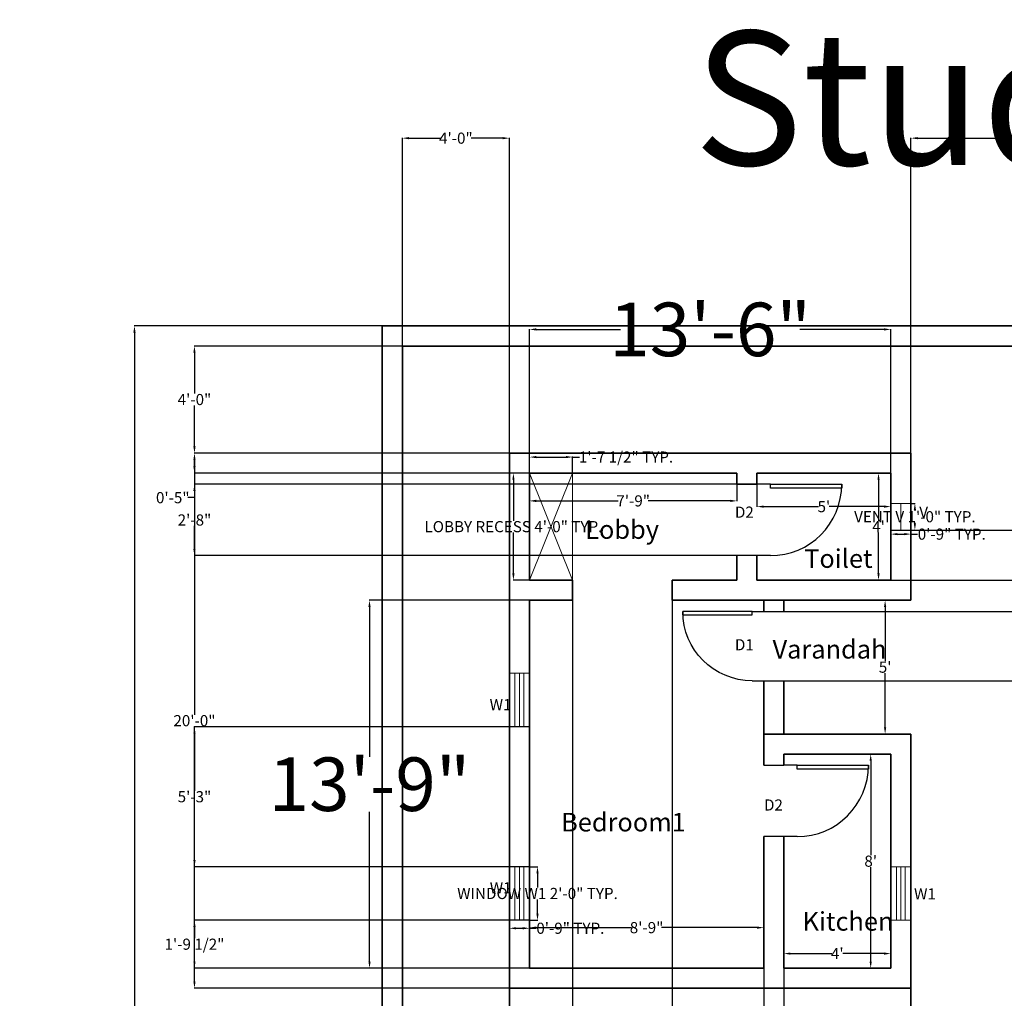
# Model space of a CAD drawing. Units: inches. Extents: x -205 to 674, y 63 to 1798.
# Tile 3 of 4: x -205 to 236, y 1359 to 1798. Entities that reach past the tile are written whole.
import ezdxf

# ---------------------------------------------------------------- set-up
doc = ezdxf.new("R2010")
doc.units = ezdxf.units.IN
doc.header["$MEASUREMENT"] = 0
doc.layers.get('0').update_dxf_attribs({"color": 70})
for name, color, linetype, lineweight in [('A-ANNO-DIMS', 240, 'Continuous', 18), ('A-ANNO-TEXT', 240, 'Continuous', 18), ('A-AREA-IDEN', 240, 'Continuous', 18), ('A-WALL', 70, 'Continuous', 35), ('A-WALL-SITE', 70, 'Continuous', 35), ('door1', 20, 'Continuous', 25), ('door2', 160, 'Continuous', 25), ('lobby', 241, 'Continuous', 18), ('ventilator1', 210, 'Continuous', 18), ('window1', 50, 'Continuous', 18)]:
    doc.layers.add(name, color=color, linetype=linetype, lineweight=lineweight)
doc.styles.get("Standard").update_dxf_attribs({"font": 'arial.ttf'})
doc.dimstyles.get("Standard").update_dxf_attribs({"dimtxt": 5, "dimasz": 3, "dimexe": 0.18, "dimexo": 0.0625, "dimgap": 0.09, "dimtad": 0, "dimtih": 1, "dimtoh": 1, "dimdec": 0, "dimzin": 0, "dimdsep": 46, "dimlunit": 3, "dimtxsty": 'Standard', "dimcen": 0.09, "dimadec": 0, "dimazin": 0, "dimtfac": 1, "dimtdec": 0, "dimtofl": 0, "dimtmove": 0, "dimatfit": 3, "dimfxl": 1, "dimtolj": 1, "dimtzin": 0, "dimarcsym": 0})

# ---------------------------------------------------------------- blocks, each defined once
blk = doc.blocks.new('*D1')
at = {"layer": 'A-ANNO-DIMS', "color": 0, "lineweight": -2, "transparency": 16777216}
for p, q in [((23.48, 1537.3), (-48.36, 1537.3)), ((-48.18, 1534.3), (-48.18, 1467.15)), ((-48.18, 1375.3), (-48.18, 1442.45)), ((23.48, 1372.3), (-48.36, 1372.3))]:
    blk.add_line(p, q, dxfattribs=at)
at = {"layer": 'A-ANNO-DIMS', "color": 0, "transparency": 16777216}
for points in [[(-48.68, 1534.3), (-47.68, 1534.3), (-48.18, 1537.3)], [(-48.68, 1375.3), (-47.68, 1375.3), (-48.18, 1372.3)]]:
    blk.add_solid(points, dxfattribs=at)
at = {"layer": 'Defpoints', "color": 0, "transparency": 16777216}
for p in [(23.54, 1537.3), (-48.18, 1372.3), (23.54, 1372.3)]:
    blk.add_point(p, dxfattribs=at)
at = {"layer": 'A-ANNO-DIMS', "color": 0, "transparency": 16777216, "insert": (-48.18, 1454.8), "char_height": 5, "attachment_point": 5}
blk.add_mtext('\\A1;{\\H4.8x;13\'-9"}', dxfattribs=at)
blk = doc.blocks.new('*D2')
at = {"layer": 'A-ANNO-DIMS', "color": 0, "lineweight": -2, "transparency": 16777216}
for p, q in [((23.54, 1594.36), (23.54, 1658.92)), ((26.54, 1658.74), (64.36, 1658.74)), ((182.54, 1658.74), (144.73, 1658.74)), ((185.54, 1594.36), (185.54, 1658.92))]:
    blk.add_line(p, q, dxfattribs=at)
at = {"layer": 'A-ANNO-DIMS', "color": 0, "transparency": 16777216}
for points in [[(26.54, 1659.24), (26.54, 1658.24), (23.54, 1658.74)], [(182.54, 1659.24), (182.54, 1658.24), (185.54, 1658.74)]]:
    blk.add_solid(points, dxfattribs=at)
at = {"layer": 'Defpoints', "color": 0, "transparency": 16777216}
for p in [(185.54, 1658.74), (23.54, 1594.3), (185.54, 1594.3)]:
    blk.add_point(p, dxfattribs=at)
at = {"layer": 'A-ANNO-DIMS', "color": 0, "transparency": 16777216, "insert": (104.54, 1658.74), "char_height": 5, "attachment_point": 5}
blk.add_mtext('\\A1;{\\H4.8x;13\'-6"}', dxfattribs=at)
blk = doc.blocks.new('*U4')
for p, q in [((0, 0), (0, -6)), ((36, 0), (36, -6))]:
    blk.add_line(p, q)
blk.add_lwpolyline([(0, 0), (0, 36), (1.75, 36), (1.75, 0)], close=True)
blk.add_arc((0, 0), 36, 0, 90)
blk = doc.blocks.new('*U5')
for p, q in [((0, 0), (0, -6)), ((32, 0), (32, -6))]:
    blk.add_line(p, q)
blk.add_lwpolyline([(0, 0), (0, 32), (1.75, 32), (1.75, 0)], close=True)
blk.add_arc((0, 0), 32, 0, 90)
blk = doc.blocks.new('*D18')
at = {"layer": 'A-ANNO-DIMS', "color": 0, "lineweight": -2, "transparency": 16777216}
for p, q in [((-42.52, 1660.3), (-153.74, 1660.3)), ((-153.56, 1657.3), (-153.56, 919.64)), ((-153.56, 157.3), (-153.56, 894.96)), ((-42.52, 154.3), (-153.74, 154.3))]:
    blk.add_line(p, q, dxfattribs=at)
at = {"layer": 'A-ANNO-DIMS', "color": 0, "transparency": 16777216}
for points in [[(-154.06, 1657.3), (-153.06, 1657.3), (-153.56, 1660.3)], [(-154.06, 157.3), (-153.06, 157.3), (-153.56, 154.3)]]:
    blk.add_solid(points, dxfattribs=at)
at = {"layer": 'Defpoints', "color": 0, "transparency": 16777216}
for p in [(-42.46, 1660.3), (-153.56, 154.3), (-42.46, 154.3)]:
    blk.add_point(p, dxfattribs=at)
at = {"layer": 'A-ANNO-DIMS', "color": 0, "transparency": 16777216, "insert": (-153.56, 907.3), "char_height": 5, "attachment_point": 5}
blk.add_mtext('\\A1;{\\H4.8x;125\'-6"}', dxfattribs=at)
blk = doc.blocks.new('*D20')
at = {"layer": 'A-ANNO-DIMS', "color": 0, "lineweight": -2, "transparency": 16777216}
for p, q in [((23.54, 1372.36), (23.54, 1390.67)), ((128.54, 1372.36), (128.54, 1390.67)), ((26.54, 1390.49), (69.3, 1390.49)), ((125.54, 1390.49), (82.78, 1390.49))]:
    blk.add_line(p, q, dxfattribs=at)
at = {"layer": 'A-ANNO-DIMS', "color": 0, "transparency": 16777216}
for points in [[(26.54, 1390.99), (26.54, 1389.99), (23.54, 1390.49)], [(125.54, 1390.99), (125.54, 1389.99), (128.54, 1390.49)]]:
    blk.add_solid(points, dxfattribs=at)
at = {"layer": 'Defpoints', "color": 0, "transparency": 16777216}
for p in [(128.54, 1390.49), (23.54, 1372.3), (128.54, 1372.3)]:
    blk.add_point(p, dxfattribs=at)
at = {"layer": 'A-ANNO-DIMS', "color": 0, "transparency": 16777216, "insert": (76.04, 1390.49), "char_height": 5, "attachment_point": 5}
blk.add_mtext('\\A1;8\'-9"', dxfattribs=at)
blk = doc.blocks.new('*D21')
at = {"layer": 'A-ANNO-DIMS', "color": 0, "lineweight": -2, "transparency": 16777216}
for p, q in [((137.54, 1372.36), (137.54, 1379.04)), ((140.54, 1378.86), (159.05, 1378.86)), ((182.54, 1378.86), (164.03, 1378.86)), ((185.54, 1372.36), (185.54, 1379.04))]:
    blk.add_line(p, q, dxfattribs=at)
at = {"layer": 'A-ANNO-DIMS', "color": 0, "transparency": 16777216}
for points in [[(140.54, 1379.36), (140.54, 1378.36), (137.54, 1378.86)], [(182.54, 1379.36), (182.54, 1378.36), (185.54, 1378.86)]]:
    blk.add_solid(points, dxfattribs=at)
at = {"layer": 'Defpoints', "color": 0, "transparency": 16777216}
for p in [(185.54, 1378.86), (137.54, 1372.3), (185.54, 1372.3)]:
    blk.add_point(p, dxfattribs=at)
at = {"layer": 'A-ANNO-DIMS', "color": 0, "transparency": 16777216, "insert": (161.54, 1378.86), "char_height": 5, "attachment_point": 5}
blk.add_mtext("\\A1;4'", dxfattribs=at)
blk = doc.blocks.new('*D22')
at = {"layer": 'A-ANNO-DIMS', "color": 0, "lineweight": -2, "transparency": 16777216}
for p, q in [((185.48, 1468.3), (176.35, 1468.3)), ((176.53, 1465.3), (176.53, 1422.94)), ((176.53, 1375.3), (176.53, 1417.66)), ((185.48, 1372.3), (176.35, 1372.3))]:
    blk.add_line(p, q, dxfattribs=at)
at = {"layer": 'A-ANNO-DIMS', "color": 0, "transparency": 16777216}
for points in [[(176.03, 1465.3), (177.03, 1465.3), (176.53, 1468.3)], [(176.03, 1375.3), (177.03, 1375.3), (176.53, 1372.3)]]:
    blk.add_solid(points, dxfattribs=at)
at = {"layer": 'Defpoints', "color": 0, "transparency": 16777216}
for p in [(185.54, 1468.3), (176.53, 1372.3), (185.54, 1372.3)]:
    blk.add_point(p, dxfattribs=at)
at = {"layer": 'A-ANNO-DIMS', "color": 0, "transparency": 16777216, "insert": (176.53, 1420.3), "char_height": 5, "attachment_point": 5}
blk.add_mtext("\\A1;8'", dxfattribs=at)
blk = doc.blocks.new('*D23')
at = {"layer": 'A-ANNO-DIMS', "color": 0, "lineweight": -2, "transparency": 16777216}
for p, q in [((185.48, 1594.3), (179.86, 1594.3)), ((180.04, 1591.3), (180.04, 1572.89)), ((180.04, 1549.3), (180.04, 1567.71)), ((185.48, 1546.3), (179.86, 1546.3))]:
    blk.add_line(p, q, dxfattribs=at)
at = {"layer": 'A-ANNO-DIMS', "color": 0, "transparency": 16777216}
for points in [[(179.54, 1591.3), (180.54, 1591.3), (180.04, 1594.3)], [(179.54, 1549.3), (180.54, 1549.3), (180.04, 1546.3)]]:
    blk.add_solid(points, dxfattribs=at)
at = {"layer": 'Defpoints', "color": 0, "transparency": 16777216}
for p in [(185.54, 1594.3), (180.04, 1546.3), (185.54, 1546.3)]:
    blk.add_point(p, dxfattribs=at)
at = {"layer": 'A-ANNO-DIMS', "color": 0, "transparency": 16777216, "insert": (180.04, 1570.3), "char_height": 5, "attachment_point": 5}
blk.add_mtext("\\A1;4'", dxfattribs=at)
blk = doc.blocks.new('*D24')
at = {"layer": 'A-ANNO-DIMS', "color": 0, "lineweight": -2, "transparency": 16777216}
for p, q in [((125.54, 1594.24), (125.54, 1579.11)), ((185.54, 1594.24), (185.54, 1579.11)), ((128.54, 1579.29), (153.15, 1579.29)), ((182.54, 1579.29), (157.93, 1579.29))]:
    blk.add_line(p, q, dxfattribs=at)
at = {"layer": 'A-ANNO-DIMS', "color": 0, "transparency": 16777216}
for points in [[(128.54, 1579.79), (128.54, 1578.79), (125.54, 1579.29)], [(182.54, 1579.79), (182.54, 1578.79), (185.54, 1579.29)]]:
    blk.add_solid(points, dxfattribs=at)
at = {"layer": 'Defpoints', "color": 0, "transparency": 16777216}
for p in [(125.54, 1594.3), (185.54, 1594.3), (125.54, 1579.29)]:
    blk.add_point(p, dxfattribs=at)
at = {"layer": 'A-ANNO-DIMS', "color": 0, "transparency": 16777216, "insert": (155.54, 1579.29), "char_height": 5, "attachment_point": 5}
blk.add_mtext("\\A1;5'", dxfattribs=at)
blk = doc.blocks.new('*D25')
at = {"layer": 'A-ANNO-DIMS', "color": 0, "lineweight": -2, "transparency": 16777216}
for p, q in [((23.54, 1594.24), (23.54, 1581.67)), ((116.54, 1594.24), (116.54, 1581.67)), ((26.54, 1581.85), (63.33, 1581.85)), ((113.54, 1581.85), (76.76, 1581.85))]:
    blk.add_line(p, q, dxfattribs=at)
at = {"layer": 'A-ANNO-DIMS', "color": 0, "transparency": 16777216}
for points in [[(26.54, 1582.35), (26.54, 1581.35), (23.54, 1581.85)], [(113.54, 1582.35), (113.54, 1581.35), (116.54, 1581.85)]]:
    blk.add_solid(points, dxfattribs=at)
at = {"layer": 'Defpoints', "color": 0, "transparency": 16777216}
for p in [(23.54, 1594.3), (116.54, 1594.3), (23.54, 1581.85)]:
    blk.add_point(p, dxfattribs=at)
at = {"layer": 'A-ANNO-DIMS', "color": 0, "transparency": 16777216, "insert": (70.04, 1581.85), "char_height": 5, "attachment_point": 5}
blk.add_mtext('\\A1;7\'-9"', dxfattribs=at)
blk = doc.blocks.new('*D26')
at = {"layer": 'A-ANNO-DIMS', "color": 0, "lineweight": -2, "transparency": 16777216}
for p, q in [((194.48, 1537.3), (182.81, 1537.3)), ((182.99, 1534.3), (182.99, 1509.93)), ((182.99, 1480.3), (182.99, 1504.67)), ((194.48, 1477.3), (182.81, 1477.3))]:
    blk.add_line(p, q, dxfattribs=at)
at = {"layer": 'A-ANNO-DIMS', "color": 0, "transparency": 16777216}
for points in [[(182.49, 1534.3), (183.49, 1534.3), (182.99, 1537.3)], [(182.49, 1480.3), (183.49, 1480.3), (182.99, 1477.3)]]:
    blk.add_solid(points, dxfattribs=at)
at = {"layer": 'Defpoints', "color": 0, "transparency": 16777216}
for p in [(194.54, 1537.3), (182.99, 1477.3), (194.54, 1477.3)]:
    blk.add_point(p, dxfattribs=at)
at = {"layer": 'A-ANNO-DIMS', "color": 0, "transparency": 16777216, "insert": (182.99, 1507.3), "char_height": 5, "attachment_point": 5}
blk.add_mtext("\\A1;5'", dxfattribs=at)
blk = doc.blocks.new('WIN-W1-24IN')
for p, q in [((2.5, 24), (2.5, 0)), ((4.5, 24), (4.5, 0)), ((6.5, 24), (6.5, 0))]:
    blk.add_line(p, q)
blk.add_lwpolyline([(0, 24), (9, 24), (9, 0), (0, 0)], close=True)
blk = doc.blocks.new('VENT-V-12IN')
blk.add_line((4.5, 12), (4.5, 0))
blk.add_lwpolyline([(9, 0), (0, 0), (0, 12), (9, 12)], close=True)
blk = doc.blocks.new('LOBBY-RECESS')
for p, q in [((0, 48), (19.36, 0)), ((0, 0), (19.36, 48)), ((19.36, 48), (19.36, 0))]:
    blk.add_line(p, q)
blk = doc.blocks.new('*D30')
at = {"layer": 'A-ANNO-DIMS', "color": 0, "lineweight": -2, "transparency": 16777216}
for p, q in [((23.6, 1417.81), (27.32, 1417.81)), ((27.14, 1414.81), (27.14, 1408.49)), ((27.14, 1396.81), (27.14, 1403.13)), ((23.6, 1393.81), (27.32, 1393.81))]:
    blk.add_line(p, q, dxfattribs=at)
at = {"layer": 'A-ANNO-DIMS', "color": 0, "transparency": 16777216}
for points in [[(26.64, 1414.81), (27.64, 1414.81), (27.14, 1417.81)], [(26.64, 1396.81), (27.64, 1396.81), (27.14, 1393.81)]]:
    blk.add_solid(points, dxfattribs=at)
at = {"layer": 'Defpoints', "color": 0, "transparency": 16777216}
for p in [(23.54, 1417.81), (27.14, 1417.81), (23.54, 1393.81)]:
    blk.add_point(p, dxfattribs=at)
at = {"layer": 'A-ANNO-DIMS', "color": 0, "transparency": 16777216, "insert": (27.14, 1405.81), "char_height": 5, "attachment_point": 5}
blk.add_mtext('\\A1;WINDOW W1 2\'-0" TYP.', dxfattribs=at)
blk = doc.blocks.new('*D31')
at = {"layer": 'A-ANNO-DIMS', "color": 0, "lineweight": -2, "transparency": 16777216}
for p, q in [((14.54, 1393.75), (14.54, 1390.03)), ((23.54, 1393.75), (23.54, 1390.03)), ((17.54, 1390.21), (20.54, 1390.21)), ((23.54, 1390.21), (26.54, 1390.21))]:
    blk.add_line(p, q, dxfattribs=at)
at = {"layer": 'A-ANNO-DIMS', "color": 0, "transparency": 16777216}
for points in [[(17.54, 1390.71), (17.54, 1389.71), (14.54, 1390.21)], [(20.54, 1390.71), (20.54, 1389.71), (23.54, 1390.21)]]:
    blk.add_solid(points, dxfattribs=at)
at = {"layer": 'Defpoints', "color": 0, "transparency": 16777216}
for p in [(14.54, 1393.81), (23.54, 1393.81), (23.54, 1390.21)]:
    blk.add_point(p, dxfattribs=at)
at = {"layer": 'A-ANNO-DIMS', "color": 0, "transparency": 16777216, "insert": (41.87, 1390.21), "char_height": 5, "attachment_point": 5}
blk.add_mtext('\\A1;0\'-9" TYP.', dxfattribs=at)
blk = doc.blocks.new('*D32')
at = {"layer": 'A-ANNO-DIMS', "color": 0, "lineweight": -2, "transparency": 16777216}
for p, q in [((194.6, 1580.75), (196.52, 1580.75)), ((196.34, 1577.75), (196.34, 1577.4)), ((196.34, 1571.75), (196.34, 1572.11)), ((194.6, 1568.75), (196.52, 1568.75))]:
    blk.add_line(p, q, dxfattribs=at)
at = {"layer": 'A-ANNO-DIMS', "color": 0, "transparency": 16777216}
for points in [[(195.84, 1577.75), (196.84, 1577.75), (196.34, 1580.75)], [(195.84, 1571.75), (196.84, 1571.75), (196.34, 1568.75)]]:
    blk.add_solid(points, dxfattribs=at)
at = {"layer": 'Defpoints', "color": 0, "transparency": 16777216}
for p in [(194.54, 1580.75), (196.34, 1580.75), (194.54, 1568.75)]:
    blk.add_point(p, dxfattribs=at)
at = {"layer": 'A-ANNO-DIMS', "color": 0, "transparency": 16777216, "insert": (196.34, 1574.75), "char_height": 5, "attachment_point": 5}
blk.add_mtext('\\A1;VENT V 1\'-0" TYP.', dxfattribs=at)
blk = doc.blocks.new('*D33')
at = {"layer": 'A-ANNO-DIMS', "color": 0, "lineweight": -2, "transparency": 16777216}
for p, q in [((185.54, 1568.69), (185.54, 1566.77)), ((194.54, 1568.69), (194.54, 1566.77)), ((188.54, 1566.95), (191.54, 1566.95)), ((194.54, 1566.95), (197.54, 1566.95))]:
    blk.add_line(p, q, dxfattribs=at)
at = {"layer": 'A-ANNO-DIMS', "color": 0, "transparency": 16777216}
for points in [[(188.54, 1567.45), (188.54, 1566.45), (185.54, 1566.95)], [(191.54, 1567.45), (191.54, 1566.45), (194.54, 1566.95)]]:
    blk.add_solid(points, dxfattribs=at)
at = {"layer": 'Defpoints', "color": 0, "transparency": 16777216}
for p in [(185.54, 1568.75), (194.54, 1568.75), (194.54, 1566.95)]:
    blk.add_point(p, dxfattribs=at)
at = {"layer": 'A-ANNO-DIMS', "color": 0, "transparency": 16777216, "insert": (212.87, 1566.95), "char_height": 5, "attachment_point": 5}
blk.add_mtext('\\A1;0\'-9" TYP.', dxfattribs=at)
blk = doc.blocks.new('*D34')
at = {"layer": 'A-ANNO-DIMS', "color": 0, "lineweight": -2, "transparency": 16777216}
for p, q in [((23.48, 1594.3), (16.16, 1594.3)), ((16.34, 1591.3), (16.34, 1572.98)), ((16.34, 1549.3), (16.34, 1567.62)), ((23.48, 1546.3), (16.16, 1546.3))]:
    blk.add_line(p, q, dxfattribs=at)
at = {"layer": 'A-ANNO-DIMS', "color": 0, "transparency": 16777216}
for points in [[(15.84, 1591.3), (16.84, 1591.3), (16.34, 1594.3)], [(15.84, 1549.3), (16.84, 1549.3), (16.34, 1546.3)]]:
    blk.add_solid(points, dxfattribs=at)
at = {"layer": 'Defpoints', "color": 0, "transparency": 16777216}
for p in [(16.34, 1594.3), (23.54, 1594.3), (23.54, 1546.3)]:
    blk.add_point(p, dxfattribs=at)
at = {"layer": 'A-ANNO-DIMS', "color": 0, "transparency": 16777216, "insert": (16.34, 1570.3), "char_height": 5, "attachment_point": 5}
blk.add_mtext('\\A1;LOBBY RECESS 4\'-0" TYP.', dxfattribs=at)
blk = doc.blocks.new('*D35')
at = {"layer": 'A-ANNO-DIMS', "color": 0, "lineweight": -2, "transparency": 16777216}
for p, q in [((23.54, 1594.36), (23.54, 1601.68)), ((26.54, 1601.5), (39.9, 1601.5)), ((42.9, 1594.36), (42.9, 1601.68)), ((42.9, 1601.5), (45.9, 1601.5))]:
    blk.add_line(p, q, dxfattribs=at)
at = {"layer": 'A-ANNO-DIMS', "color": 0, "transparency": 16777216}
for points in [[(26.54, 1602), (26.54, 1601), (23.54, 1601.5)], [(39.9, 1602), (39.9, 1601), (42.9, 1601.5)]]:
    blk.add_solid(points, dxfattribs=at)
at = {"layer": 'Defpoints', "color": 0, "transparency": 16777216}
for p in [(42.9, 1601.5), (23.54, 1594.3), (42.9, 1594.3)]:
    blk.add_point(p, dxfattribs=at)
at = {"layer": 'A-ANNO-DIMS', "color": 0, "transparency": 16777216, "insert": (66.82, 1601.5), "char_height": 5, "attachment_point": 5}
blk.add_mtext('\\A1;1\'-7 1/2" TYP.', dxfattribs=at)
blk = doc.blocks.new('*D36')
at = {"layer": 'A-ANNO-DIMS', "color": 0, "lineweight": -2, "transparency": 16777216}
for p, q in [((-33.46, 1651.36), (-33.46, 1744.68)), ((-30.46, 1744.5), (-16.29, 1744.5)), ((11.54, 1744.5), (-2.62, 1744.5)), ((14.54, 1603.36), (14.54, 1744.68))]:
    blk.add_line(p, q, dxfattribs=at)
at = {"layer": 'A-ANNO-DIMS', "color": 0, "transparency": 16777216}
for points in [[(-30.46, 1745), (-30.46, 1744), (-33.46, 1744.5)], [(11.54, 1745), (11.54, 1744), (14.54, 1744.5)]]:
    blk.add_solid(points, dxfattribs=at)
at = {"layer": 'Defpoints', "color": 0, "transparency": 16777216}
for p in [(14.54, 1744.5), (-33.46, 1651.3), (14.54, 1603.3)]:
    blk.add_point(p, dxfattribs=at)
at = {"layer": 'A-ANNO-DIMS', "color": 0, "transparency": 16777216, "insert": (-9.46, 1744.5), "char_height": 5, "attachment_point": 5}
blk.add_mtext('\\A1;4\'-0"', dxfattribs=at)
blk = doc.blocks.new('*D37')
at = {"layer": 'A-ANNO-DIMS', "color": 0, "lineweight": -2, "transparency": 16777216}
for p, q in [((194.54, 1603.36), (194.54, 1744.68)), ((197.54, 1744.5), (258.1, 1744.5)), ((335.54, 1744.5), (274.99, 1744.5)), ((338.54, 1603.36), (338.54, 1744.68))]:
    blk.add_line(p, q, dxfattribs=at)
at = {"layer": 'A-ANNO-DIMS', "color": 0, "transparency": 16777216}
for points in [[(197.54, 1745), (197.54, 1744), (194.54, 1744.5)], [(335.54, 1745), (335.54, 1744), (338.54, 1744.5)]]:
    blk.add_solid(points, dxfattribs=at)
at = {"layer": 'Defpoints', "color": 0, "transparency": 16777216}
for p in [(338.54, 1744.5), (194.54, 1603.3), (338.54, 1603.3)]:
    blk.add_point(p, dxfattribs=at)
at = {"layer": 'A-ANNO-DIMS', "color": 0, "transparency": 16777216, "insert": (266.54, 1744.5), "char_height": 5, "attachment_point": 5}
blk.add_mtext('\\A1;12\'-0"', dxfattribs=at)
blk = doc.blocks.new('*D38')
at = {"layer": 'A-ANNO-DIMS', "color": 0, "lineweight": -2, "transparency": 16777216}
for p, q in [((-33.52, 1651.3), (-126.84, 1651.3)), ((-126.66, 1648.3), (-126.66, 1629.94)), ((-126.66, 1606.3), (-126.66, 1624.66)), ((14.48, 1603.3), (-126.84, 1603.3))]:
    blk.add_line(p, q, dxfattribs=at)
at = {"layer": 'A-ANNO-DIMS', "color": 0, "transparency": 16777216}
for points in [[(-127.16, 1648.3), (-126.16, 1648.3), (-126.66, 1651.3)], [(-127.16, 1606.3), (-126.16, 1606.3), (-126.66, 1603.3)]]:
    blk.add_solid(points, dxfattribs=at)
at = {"layer": 'Defpoints', "color": 0, "transparency": 16777216}
for p in [(-33.46, 1651.3), (-126.66, 1603.3), (14.54, 1603.3)]:
    blk.add_point(p, dxfattribs=at)
at = {"layer": 'A-ANNO-DIMS', "color": 0, "transparency": 16777216, "insert": (-126.66, 1627.3), "char_height": 5, "attachment_point": 5}
blk.add_mtext('\\A1;4\'-0"', dxfattribs=at)
blk = doc.blocks.new('*D39')
at = {"layer": 'A-ANNO-DIMS', "color": 0, "lineweight": -2, "transparency": 16777216}
for p, q in [((14.48, 1603.3), (-126.84, 1603.3)), ((-126.66, 1600.3), (-126.66, 1485.94)), ((-126.66, 1366.3), (-126.66, 1480.66)), ((14.48, 1363.3), (-126.84, 1363.3))]:
    blk.add_line(p, q, dxfattribs=at)
at = {"layer": 'A-ANNO-DIMS', "color": 0, "transparency": 16777216}
for points in [[(-127.16, 1600.3), (-126.16, 1600.3), (-126.66, 1603.3)], [(-127.16, 1366.3), (-126.16, 1366.3), (-126.66, 1363.3)]]:
    blk.add_solid(points, dxfattribs=at)
at = {"layer": 'Defpoints', "color": 0, "transparency": 16777216}
for p in [(14.54, 1603.3), (-126.66, 1363.3), (14.54, 1363.3)]:
    blk.add_point(p, dxfattribs=at)
at = {"layer": 'A-ANNO-DIMS', "color": 0, "transparency": 16777216, "insert": (-126.66, 1483.3), "char_height": 5, "attachment_point": 5}
blk.add_mtext('\\A1;20\'-0"', dxfattribs=at)
blk = doc.blocks.new('*D40')
at = {"layer": 'A-ANNO-DIMS', "color": 0, "lineweight": -2, "transparency": 16777216}
for p, q in [((128.54, 1372.24), (128.54, 69.92)), ((137.54, 1372.24), (137.54, 69.92)), ((131.54, 70.1), (134.54, 70.1)), ((137.54, 70.1), (140.54, 70.1))]:
    blk.add_line(p, q, dxfattribs=at)
at = {"layer": 'A-ANNO-DIMS', "color": 0, "transparency": 16777216}
for points in [[(131.54, 70.6), (131.54, 69.6), (128.54, 70.1)], [(134.54, 70.6), (134.54, 69.6), (137.54, 70.1)]]:
    blk.add_solid(points, dxfattribs=at)
at = {"layer": 'Defpoints', "color": 0, "transparency": 16777216}
for p in [(128.54, 1372.3), (137.54, 1372.3), (137.54, 70.1)]:
    blk.add_point(p, dxfattribs=at)
at = {"layer": 'A-ANNO-DIMS', "color": 0, "transparency": 16777216, "insert": (147.28, 70.1), "char_height": 5, "attachment_point": 5}
blk.add_mtext('\\A1;0\'-9"', dxfattribs=at)
blk = doc.blocks.new('*D41')
at = {"layer": 'A-ANNO-DIMS', "color": 0, "lineweight": -2, "transparency": 16777216}
for p, q in [((23.48, 1393.81), (-126.84, 1393.81)), ((-126.66, 1390.81), (-126.66, 1385.73)), ((-126.66, 1375.3), (-126.66, 1380.38)), ((23.48, 1372.3), (-126.84, 1372.3))]:
    blk.add_line(p, q, dxfattribs=at)
at = {"layer": 'A-ANNO-DIMS', "color": 0, "transparency": 16777216}
for points in [[(-127.16, 1390.81), (-126.16, 1390.81), (-126.66, 1393.81)], [(-127.16, 1375.3), (-126.16, 1375.3), (-126.66, 1372.3)]]:
    blk.add_solid(points, dxfattribs=at)
at = {"layer": 'Defpoints', "color": 0, "transparency": 16777216}
for p in [(-126.66, 1393.81), (23.54, 1393.81), (23.54, 1372.3)]:
    blk.add_point(p, dxfattribs=at)
at = {"layer": 'A-ANNO-DIMS', "color": 0, "transparency": 16777216, "insert": (-126.66, 1383.05), "char_height": 5, "attachment_point": 5}
blk.add_mtext('\\A1;1\'-9 1/2"', dxfattribs=at)
blk = doc.blocks.new('*D42')
at = {"layer": 'A-ANNO-DIMS', "color": 0, "lineweight": -2, "transparency": 16777216}
for p, q in [((23.48, 1480.57), (-126.84, 1480.57)), ((-126.66, 1477.57), (-126.66, 1451.84)), ((-126.66, 1420.81), (-126.66, 1446.55)), ((23.48, 1417.81), (-126.84, 1417.81))]:
    blk.add_line(p, q, dxfattribs=at)
at = {"layer": 'A-ANNO-DIMS', "color": 0, "transparency": 16777216}
for points in [[(-127.16, 1477.57), (-126.16, 1477.57), (-126.66, 1480.57)], [(-127.16, 1420.81), (-126.16, 1420.81), (-126.66, 1417.81)]]:
    blk.add_solid(points, dxfattribs=at)
at = {"layer": 'Defpoints', "color": 0, "transparency": 16777216}
for p in [(-126.66, 1480.57), (23.54, 1480.57), (23.54, 1417.81)]:
    blk.add_point(p, dxfattribs=at)
at = {"layer": 'A-ANNO-DIMS', "color": 0, "transparency": 16777216, "insert": (-126.66, 1449.19), "char_height": 5, "attachment_point": 5}
blk.add_mtext('\\A1;5\'-3"', dxfattribs=at)
blk = doc.blocks.new('*D43')
at = {"layer": 'A-ANNO-DIMS', "color": 0, "lineweight": -2, "transparency": 16777216}
for p, q in [((185.6, 1568.75), (659.92, 1568.75)), ((659.74, 1565.75), (659.74, 1560.2)), ((659.74, 1549.3), (659.74, 1554.85)), ((185.6, 1546.3), (659.92, 1546.3))]:
    blk.add_line(p, q, dxfattribs=at)
at = {"layer": 'A-ANNO-DIMS', "color": 0, "transparency": 16777216}
for points in [[(659.24, 1565.75), (660.24, 1565.75), (659.74, 1568.75)], [(659.24, 1549.3), (660.24, 1549.3), (659.74, 1546.3)]]:
    blk.add_solid(points, dxfattribs=at)
at = {"layer": 'Defpoints', "color": 0, "transparency": 16777216}
for p in [(185.54, 1568.75), (659.74, 1568.75), (185.54, 1546.3)]:
    blk.add_point(p, dxfattribs=at)
at = {"layer": 'A-ANNO-DIMS', "color": 0, "transparency": 16777216, "insert": (659.74, 1557.53), "char_height": 5, "attachment_point": 5}
blk.add_mtext('\\A1;1\'-10 1/2"', dxfattribs=at)
blk = doc.blocks.new('*D44')
at = {"layer": 'A-ANNO-DIMS', "color": 0, "lineweight": -2, "transparency": 16777216}
for p, q in [((137.6, 1532.3), (659.92, 1532.3)), ((659.74, 1529.3), (659.74, 1519.35)), ((659.74, 1504.19), (659.74, 1514.15)), ((137.6, 1501.19), (659.92, 1501.19))]:
    blk.add_line(p, q, dxfattribs=at)
at = {"layer": 'A-ANNO-DIMS', "color": 0, "transparency": 16777216}
for points in [[(659.24, 1529.3), (660.24, 1529.3), (659.74, 1532.3)], [(659.24, 1504.19), (660.24, 1504.19), (659.74, 1501.19)]]:
    blk.add_solid(points, dxfattribs=at)
at = {"layer": 'Defpoints', "color": 0, "transparency": 16777216}
for p in [(137.54, 1532.3), (137.54, 1501.19), (659.74, 1501.19)]:
    blk.add_point(p, dxfattribs=at)
at = {"layer": 'A-ANNO-DIMS', "color": 0, "transparency": 16777216, "insert": (659.74, 1516.75), "char_height": 5, "attachment_point": 5}
blk.add_mtext('\\A1;2\'-7"', dxfattribs=at)
blk = doc.blocks.new('*D45')
at = {"layer": 'A-ANNO-DIMS', "color": 0, "lineweight": -2, "transparency": 16777216}
for p, q in [((125.48, 1589.3), (-126.84, 1589.3)), ((-126.66, 1586.3), (-126.66, 1575.94)), ((-126.66, 1560.3), (-126.66, 1570.66)), ((125.48, 1557.3), (-126.84, 1557.3))]:
    blk.add_line(p, q, dxfattribs=at)
at = {"layer": 'A-ANNO-DIMS', "color": 0, "transparency": 16777216}
for points in [[(-127.16, 1586.3), (-126.16, 1586.3), (-126.66, 1589.3)], [(-127.16, 1560.3), (-126.16, 1560.3), (-126.66, 1557.3)]]:
    blk.add_solid(points, dxfattribs=at)
at = {"layer": 'Defpoints', "color": 0, "transparency": 16777216}
for p in [(125.54, 1589.3), (-126.66, 1557.3), (125.54, 1557.3)]:
    blk.add_point(p, dxfattribs=at)
at = {"layer": 'A-ANNO-DIMS', "color": 0, "transparency": 16777216, "insert": (-126.66, 1573.3), "char_height": 5, "attachment_point": 5}
blk.add_mtext('\\A1;2\'-8"', dxfattribs=at)
blk = doc.blocks.new('*D46')
at = {"layer": 'A-ANNO-DIMS', "color": 0, "lineweight": -2, "transparency": 16777216}
for p, q in [((-126.66, 1597.3), (-126.66, 1600.3)), ((116.48, 1594.3), (-126.84, 1594.3)), ((116.48, 1589.3), (-126.84, 1589.3)), ((-126.66, 1586.3), (-126.66, 1583.3)), ((-126.66, 1583.3), (-129.66, 1583.3))]:
    blk.add_line(p, q, dxfattribs=at)
at = {"layer": 'A-ANNO-DIMS', "color": 0, "transparency": 16777216}
for points in [[(-127.16, 1597.3), (-126.16, 1597.3), (-126.66, 1594.3)], [(-127.16, 1586.3), (-126.16, 1586.3), (-126.66, 1589.3)]]:
    blk.add_solid(points, dxfattribs=at)
at = {"layer": 'Defpoints', "color": 0, "transparency": 16777216}
for p in [(116.54, 1594.3), (-126.66, 1589.3), (116.54, 1589.3)]:
    blk.add_point(p, dxfattribs=at)
at = {"layer": 'A-ANNO-DIMS', "color": 0, "transparency": 16777216, "insert": (-136.39, 1583.3), "char_height": 5, "attachment_point": 5}
blk.add_mtext('\\A1;0\'-5"', dxfattribs=at)
blk = doc.blocks.new('*D47')
at = {"layer": 'A-ANNO-DIMS', "color": 0, "lineweight": -2, "transparency": 16777216}
for p, q in [((42.9, 1546.24), (42.9, 69.92)), ((87.49, 1546.24), (87.49, 69.92)), ((45.9, 70.1), (52.64, 70.1)), ((84.49, 70.1), (77.76, 70.1))]:
    blk.add_line(p, q, dxfattribs=at)
at = {"layer": 'A-ANNO-DIMS', "color": 0, "transparency": 16777216}
for points in [[(45.9, 70.6), (45.9, 69.6), (42.9, 70.1)], [(84.49, 70.6), (84.49, 69.6), (87.49, 70.1)]]:
    blk.add_solid(points, dxfattribs=at)
at = {"layer": 'Defpoints', "color": 0, "transparency": 16777216}
for p in [(42.9, 1546.3), (87.49, 1546.3), (87.49, 70.1)]:
    blk.add_point(p, dxfattribs=at)
at = {"layer": 'A-ANNO-DIMS', "color": 0, "transparency": 16777216, "insert": (65.2, 70.1), "char_height": 5, "attachment_point": 5}
blk.add_mtext('\\A1;3\'-8 1/2"', dxfattribs=at)

msp = doc.modelspace()

# ---------------------------------------------------------------- linework, layer by layer
at = {"layer": 'A-WALL'}
for p, q in [((14.54, 1603.3), (194.54, 1603.3)), ((14.54, 1363.3), (14.54, 1603.3)), ((194.54, 1603.3), (194.54, 1537.3)), ((23.54, 1594.3), (116.54, 1594.3)), ((23.54, 1546.3), (23.54, 1594.3)), ((116.54, 1594.3), (116.54, 1589.3)), ((116.54, 1589.3), (116.54, 1594.3)), ((125.54, 1594.3), (125.54, 1589.3)), ((125.54, 1594.3), (185.54, 1594.3)), ((125.54, 1594.3), (125.54, 1589.3)), ((185.54, 1594.3), (185.54, 1546.3)), ((116.54, 1557.3), (116.54, 1546.3)), ((125.54, 1557.3), (125.54, 1546.3)), ((23.54, 1546.3), (42.9, 1546.3)), ((42.9, 1546.3), (42.9, 1537.3)), ((87.49, 1546.3), (87.49, 1537.3)), ((87.49, 1546.3), (116.54, 1546.3)), ((125.54, 1546.3), (185.54, 1546.3)), ((23.54, 1372.3), (23.54, 1537.3)), ((23.54, 1537.3), (42.9, 1537.3)), ((42.9, 1537.3), (42.9, 1537.3)), ((87.49, 1537.3), (87.49, 1537.3)), ((87.49, 1537.3), (194.54, 1537.3)), ((128.54, 1537.3), (128.54, 1532.3)), ((137.54, 1537.3), (137.54, 1532.3)), ((137.55, 1537.29), (137.55, 1532.4)), ((128.54, 1501.19), (128.54, 1463.3)), ((137.54, 1501.19), (137.54, 1477.3)), ((194.54, 1477.3), (128.54, 1477.3)), ((194.54, 1477.3), (194.54, 1363.3)), ((128.54, 1463.3), (128.54, 1468.3)), ((185.54, 1468.3), (137.54, 1468.3)), ((137.54, 1468.3), (137.54, 1463.3)), ((137.54, 1468.3), (137.54, 1463.3)), ((185.54, 1468.3), (185.54, 1372.3)), ((128.54, 1431.3), (128.54, 1372.3)), ((137.54, 1431.3), (137.54, 1372.3)), ((137.54, 1431.3), (137.54, 1372.3)), ((128.54, 1372.3), (23.54, 1372.3)), ((185.54, 1372.3), (137.54, 1372.3)), ((194.54, 1363.3), (14.54, 1363.3)), ((194.54, 1363.3), (14.54, 1363.3)), ((14.54, 1363.3), (14.54, 1123.3)), ((194.54, 1249.3), (194.54, 1363.3))]:
    msp.add_line(p, q, dxfattribs=at)
at = {"layer": 'A-WALL-SITE'}
for points in [[(575.54, 154.3), (575.54, 1660.3), (266.54, 1660.3), (-42.46, 1660.3), (-42.46, 154.3), (266.54, 154.3)], [(566.54, 163.3), (566.54, 1651.3), (266.54, 1651.3), (-33.46, 1651.3), (-33.46, 163.3), (266.54, 163.3)]]:
    msp.add_lwpolyline(points, close=True, dxfattribs=at)
at = {"layer": 'door1'}
for p, q in [((128.54, 1532.3), (137.54, 1532.3)), ((128.54, 1501.19), (137.54, 1501.19))]:
    msp.add_line(p, q, dxfattribs=at)
at = {"layer": 'door2'}
for p, q in [((116.54, 1589.3), (125.54, 1589.3)), ((125.54, 1557.3), (116.54, 1557.3)), ((128.54, 1463.3), (137.54, 1463.3)), ((137.54, 1431.3), (128.54, 1431.3))]:
    msp.add_line(p, q, dxfattribs=at)

# ---------------------------------------------------------------- block references
at = {"layer": 'door1', "xscale": -0.8640557789234337, "yscale": 0.8640557789234337, "zscale": 0.8640557789234337, "rotation": 90}
msp.add_blockref('*U4', (123.36, 1532.3), dxfattribs=at)
at = {"layer": 'door2', "rotation": 270}
for p in [(131.54, 1589.3), (143.54, 1463.3)]:
    msp.add_blockref('*U5', p, dxfattribs=at)
at = {"layer": 'lobby'}
msp.add_blockref('LOBBY-RECESS', (23.54, 1546.3), dxfattribs=at)
at = {"layer": 'ventilator1'}
msp.add_blockref('VENT-V-12IN', (185.54, 1568.75), dxfattribs=at)
at = {"layer": 'window1'}
for p in [(14.54, 1480.57), (14.54, 1393.81), (185.54, 1393.81)]:
    msp.add_blockref('WIN-W1-24IN', p, dxfattribs=at)

# ---------------------------------------------------------------- texts
at = {"layer": 'A-ANNO-TEXT', "attachment_point": 1}
for s, width, insert, char_height in [('Studio units', 509.5824, (97.11, 1792.47), 60), ('D2', 13.5017, (115.64, 1579.29), 5), ('V', 13.5017, (198.3, 1579.29), 5), ('D1', 13.5017, (115.64, 1519.84), 5), ('W1', 13.5017, (5.68, 1492.96), 5), ('D2', 13.5017, (128.68, 1447.99), 5), ('W1', 13.5017, (5.74, 1410.83), 5), ('W1', 13.5017, (195.97, 1408.11), 5)]:
    msp.add_mtext_dynamic_manual_height_columns(s, width=width, gutter_width=1, heights=[0], dxfattribs=dict(at, insert=insert, char_height=char_height))
at = {"layer": 'A-AREA-IDEN', "char_height": 8.34, "attachment_point": 1}
for s, insert in [('Lobby', (48.54, 1573.17)), ('Toilet', (146.71, 1560.16)), ('Varandah', (132.52, 1519.49)), ('Bedroom1', (37.73, 1441.95)), ('Kitchen', (145.99, 1397.47))]:
    msp.add_mtext_dynamic_manual_height_columns(s, width=37.3149, gutter_width=1.67, heights=[0], dxfattribs=dict(at, insert=insert))

# ---------------------------------------------------------------- dimensions: what is measured, and where the dimension line sits
at = {"layer": 'A-ANNO-DIMS'}
for base, p1, p2, override, picture, middle in [((14.54, 1744.5), (-33.46, 1651.3), (14.54, 1603.3), {"dimdec": 1, "dimlfac": 1, "dimrnd": 0, "dimzin": 1, "dimdsep": 46, "dimlunit": 4, "dimfrac": 2}, '*D36', (-9.46, 1744.5)), ((338.54, 1744.5), (194.54, 1603.3), (338.54, 1603.3), {"dimdec": 1, "dimlfac": 1, "dimrnd": 0, "dimzin": 1, "dimdsep": 46, "dimlunit": 4, "dimfrac": 2}, '*D37', (266.54, 1744.5)), ((23.54, 1581.85), (116.54, 1594.3), (23.54, 1594.3), {"dimclrd": 0, "dimclre": 0, "dimclrt": 0}, '*D25', (70.04, 1581.85)), ((125.54, 1579.29), (185.54, 1594.3), (125.54, 1594.3), {"dimclrd": 0, "dimclre": 0, "dimclrt": 0}, '*D24', (155.54, 1579.29)), ((87.49, 70.1), (42.9, 1546.3), (87.49, 1546.3), {"dimdec": 1, "dimlfac": 1, "dimrnd": 0, "dimzin": 1, "dimdsep": 46, "dimlunit": 4, "dimfrac": 2}, '*D47', (65.2, 70.1)), ((128.54, 1390.49), (23.54, 1372.3), (128.54, 1372.3), {"dimclrd": 0, "dimclre": 0, "dimclrt": 0}, '*D20', (76.04, 1390.49)), ((185.54, 1378.86), (137.54, 1372.3), (185.54, 1372.3), {"dimclrd": 0, "dimclre": 0, "dimclrt": 0}, '*D21', (161.54, 1378.86)), ((137.54, 70.1), (128.54, 1372.3), (137.54, 1372.3), {"dimdec": 1, "dimlfac": 1, "dimrnd": 0, "dimzin": 1, "dimdsep": 46, "dimlunit": 4, "dimfrac": 2}, '*D40', (147.28, 70.1))]:
    dim = msp.add_linear_dim(base=base, p1=p1, p2=p2, dimstyle='Standard', override=override, dxfattribs=at)
    dim.commit()
    dim.dimension.update_dxf_attribs({"geometry": picture, "text_midpoint": middle})
for base, p1, p2, text, override, picture, middle in [((185.54, 1658.74), (23.54, 1594.3), (185.54, 1594.3), '{\\H4.8x;<>}', {"dimclrd": 0, "dimclre": 0, "dimclrt": 0}, '*D2', (104.54, 1658.74)), ((42.9, 1601.5), (23.54, 1594.3), (42.9, 1594.3), '<> TYP.', {"dimdec": 1, "dimlfac": 1, "dimrnd": 0, "dimzin": 1, "dimdsep": 46, "dimlunit": 4, "dimfrac": 2}, '*D35', (66.82, 1601.5)), ((194.54, 1566.95), (185.54, 1568.75), (194.54, 1568.75), '<> TYP.', {"dimdec": 1, "dimlfac": 1, "dimrnd": 0, "dimzin": 1, "dimdsep": 46, "dimlunit": 4, "dimfrac": 2}, '*D33', (212.87, 1566.95)), ((23.54, 1390.21), (14.54, 1393.81), (23.54, 1393.81), '<> TYP.', {"dimdec": 1, "dimlfac": 1, "dimrnd": 0, "dimzin": 1, "dimdsep": 46, "dimlunit": 4, "dimfrac": 2}, '*D31', (41.87, 1390.21))]:
    dim = msp.add_linear_dim(base=base, p1=p1, p2=p2, text=text, dimstyle='Standard', override=override, dxfattribs=at)
    dim.commit()
    dim.dimension.update_dxf_attribs({"geometry": picture, "text_midpoint": middle})
for base, p1, p2, text, override, picture, middle in [((-153.56, 154.3), (-42.46, 1660.3), (-42.46, 154.3), '{\\H4.8x;<>}', {"dimclrd": 0, "dimclre": 0, "dimclrt": 0}, '*D18', (-153.56, 907.3)), ((16.34, 1594.3), (23.54, 1546.3), (23.54, 1594.3), 'LOBBY RECESS <> TYP.', {"dimdec": 1, "dimlfac": 1, "dimrnd": 0, "dimzin": 1, "dimdsep": 46, "dimlunit": 4, "dimfrac": 2}, '*D34', (16.34, 1570.3)), ((196.34, 1580.75), (194.54, 1568.75), (194.54, 1580.75), 'VENT V <> TYP.', {"dimdec": 1, "dimlfac": 1, "dimrnd": 0, "dimzin": 1, "dimdsep": 46, "dimlunit": 4, "dimfrac": 2}, '*D32', (196.34, 1574.75)), ((-48.18, 1372.3), (23.54, 1537.3), (23.54, 1372.3), '{\\H4.8x;<>}', {"dimclrd": 0, "dimclre": 0, "dimclrt": 0}, '*D1', (-48.18, 1454.8)), ((27.14, 1417.81), (23.54, 1393.81), (23.54, 1417.81), 'WINDOW W1 <> TYP.', {"dimdec": 1, "dimlfac": 1, "dimrnd": 0, "dimzin": 1, "dimdsep": 46, "dimlunit": 4, "dimfrac": 2}, '*D30', (27.14, 1405.81))]:
    dim = msp.add_linear_dim(base=base, p1=p1, p2=p2, angle=90, text=text, dimstyle='Standard', override=override, dxfattribs=at)
    dim.commit()
    dim.dimension.update_dxf_attribs({"geometry": picture, "text_midpoint": middle})
for base, p1, p2, override, picture, middle in [((-126.66, 1603.3), (-33.46, 1651.3), (14.54, 1603.3), {"dimdec": 1, "dimlfac": 1, "dimrnd": 0, "dimzin": 1, "dimdsep": 46, "dimlunit": 4, "dimfrac": 2}, '*D38', (-126.66, 1627.3)), ((-126.66, 1363.3), (14.54, 1603.3), (14.54, 1363.3), {"dimdec": 1, "dimlfac": 1, "dimrnd": 0, "dimzin": 1, "dimdsep": 46, "dimlunit": 4, "dimfrac": 2}, '*D39', (-126.66, 1483.3)), ((-126.66, 1589.3), (116.54, 1594.3), (116.54, 1589.3), {"dimdec": 1, "dimlfac": 1, "dimrnd": 0, "dimzin": 1, "dimdsep": 46, "dimlunit": 4, "dimfrac": 2}, '*D46', (-136.39, 1583.3)), ((180.04, 1546.3), (185.54, 1594.3), (185.54, 1546.3), {"dimclrd": 0, "dimclre": 0, "dimclrt": 0}, '*D23', (180.04, 1570.3)), ((-126.66, 1557.3), (125.54, 1589.3), (125.54, 1557.3), {"dimdec": 1, "dimlfac": 1, "dimrnd": 0, "dimzin": 1, "dimdsep": 46, "dimlunit": 4, "dimfrac": 2}, '*D45', (-126.66, 1573.3)), ((659.7424, 1568.7532), (185.5424, 1546.2998), (185.5424, 1568.7532), {"dimdec": 1, "dimlfac": 1, "dimrnd": 0, "dimzin": 1, "dimdsep": 46, "dimlunit": 4, "dimfrac": 2}, '*D43', (659.7424, 1557.5265)), ((182.99, 1477.3), (194.54, 1537.3), (194.54, 1477.3), {"dimclrd": 0, "dimclre": 0, "dimclrt": 0}, '*D26', (182.99, 1507.3)), ((659.74, 1501.19), (137.54, 1532.3), (137.54, 1501.19), {"dimdec": 1, "dimlfac": 1, "dimrnd": 0, "dimzin": 1, "dimdsep": 46, "dimlunit": 4, "dimfrac": 2}, '*D44', (659.74, 1516.75)), ((-126.66, 1480.57), (23.54, 1417.81), (23.54, 1480.57), {"dimdec": 1, "dimlfac": 1, "dimrnd": 0, "dimzin": 1, "dimdsep": 46, "dimlunit": 4, "dimfrac": 2}, '*D42', (-126.66, 1449.19)), ((176.53, 1372.3), (185.54, 1468.3), (185.54, 1372.3), {"dimclrd": 0, "dimclre": 0, "dimclrt": 0}, '*D22', (176.53, 1420.3)), ((-126.66, 1393.81), (23.54, 1372.3), (23.54, 1393.81), {"dimdec": 1, "dimlfac": 1, "dimrnd": 0, "dimzin": 1, "dimdsep": 46, "dimlunit": 4, "dimfrac": 2}, '*D41', (-126.66, 1383.05))]:
    dim = msp.add_linear_dim(base=base, p1=p1, p2=p2, angle=90, dimstyle='Standard', override=override, dxfattribs=at)
    dim.commit()
    dim.dimension.update_dxf_attribs({"geometry": picture, "text_midpoint": middle})

doc.saveas('drawing.dxf')
